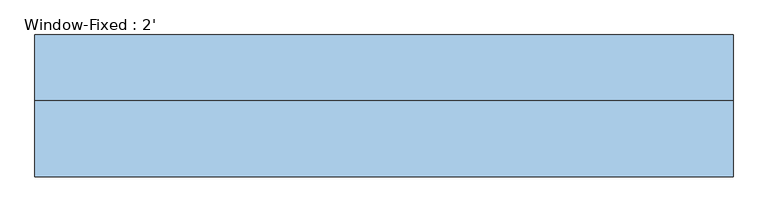
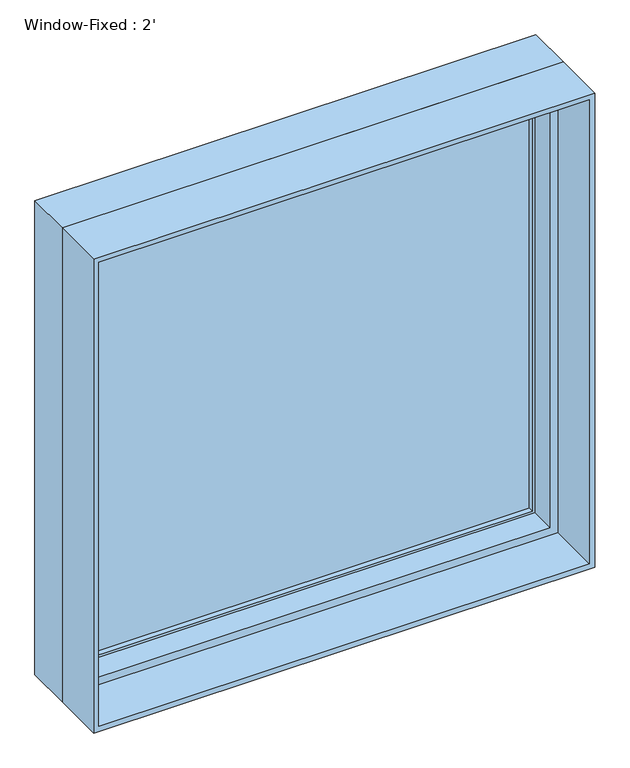
"""IFC4 building model written with IfcOpenShell, lengths in millimetres: window geometry, Window-Fixed : 2'."""

from ifc_helpers import new_model, si_unit, frame, origin, place, context, project, spatial, polyline, outline, extrude, faceted_brep, source, transform, mapped, element, save


def window_fixed_2_d4a0c5b4(model_context):
    return source(origin(), model_context, "Body", "SolidModel", [
        faceted_brep([(609.6, 19.05, 2133.6), (609.6, 133.35, 2133.6), (-609.6, 133.35, 2133.6), (-609.6, 19.05, 2133.6), (-609.6, 133.35, 914.4), (-609.6, 19.05, 914.4), (609.6, 133.35, 914.4), (609.6, 19.05, 914.4), (577.85, 19.05, 2101.85), (577.85, 19.05, 946.15), (-577.85, 19.05, 946.15), (-577.85, 19.05, 2101.85), (-596.9, 133.35, 2120.9), (-596.9, 133.35, 927.1), (596.9, 133.35, 927.1), (596.9, 133.35, 2120.9), (577.85, 82.55, 2101.85), (-577.85, 82.55, 2101.85), (596.9, 82.55, 2120.9), (-596.9, 82.55, 2120.9), (-577.85, 82.55, 946.15), (-596.9, 82.55, 927.1), (577.85, 82.55, 946.15), (596.9, 82.55, 927.1)], [[[0, 1, 2, 3]], [[3, 2, 4, 5]], [[5, 4, 6, 7]], [[3, 5, 7, 0], [8, 9, 10, 11]], [[7, 6, 1, 0]], [[1, 6, 4, 2], [12, 13, 14, 15]], [[16, 8, 11, 17]], [[15, 18, 19, 12]], [[17, 11, 10, 20]], [[12, 19, 21, 13]], [[20, 10, 9, 22]], [[13, 21, 23, 14]], [[22, 9, 8, 16]], [[18, 23, 21, 19], [17, 20, 22, 16]], [[14, 23, 18, 15]]]),
        extrude(outline(polyline([(2133.6, -609.6), (914.4, -609.6), (914.4, 609.6), (2133.6, 609.6), (2133.6, -609.6)]), holes=[polyline([(2120.9, 596.9), (927.1, 596.9), (927.1, -596.9), (2120.9, -596.9), (2120.9, 596.9)])]), frame((0.0, -114.3, 0.0), z_axis=(0.0, 1.0, 0.0), x_axis=(0.0, 0.0, 1.0)), (0.0, 0.0, 1.0), 133.35),
        extrude(outline(polyline([(927.1, 596.9), (2120.9, 596.9), (2120.9, -596.9), (927.1, -596.9), (927.1, 596.9)]), holes=[polyline([(952.5, -571.5), (2095.5, -571.5), (2095.5, 571.5), (952.5, 571.5), (952.5, -571.5)])]), frame((0.0, 82.55, 0.0), z_axis=(0.0, 1.0, 0.0), x_axis=(0.0, 0.0, 1.0)), (0.0, 0.0, 1.0), 44.45),
        extrude(outline(polyline([(571.5, 114.3), (571.5, 107.95), (-571.5, 107.95), (-571.5, 114.3), (571.5, 114.3)])), frame((0.0, 0.0, 952.5), z_axis=(0.0, 0.0, 1.0), x_axis=(1.0, 0.0, 0.0)), (0.0, 0.0, 1.0), 1143.0),
        extrude(outline(polyline([(-571.5, 95.25), (-571.5, 101.6), (571.5, 101.6), (571.5, 95.25), (-571.5, 95.25)])), frame((0.0, 0.0, 952.5), z_axis=(0.0, 0.0, 1.0), x_axis=(1.0, 0.0, 0.0)), (0.0, 0.0, 1.0), 1143.0),
    ])


if __name__ == "__main__":
    model = new_model("IFC4")
    model_context = context("Model", 3, world=origin())
    ifc_project = project(units=[si_unit("LENGTHUNIT", "METRE", prefix="MILLI")], contexts=[model_context])
    site = spatial("IfcSite", under=ifc_project)
    building = spatial("IfcBuilding", under=site)
    placement = place(None, origin())
    window_fixed_2_shape = window_fixed_2_d4a0c5b4(model_context)
    element("IfcWindow", 1, ObjectType="Window-Fixed : 2'", at=placement, inside=building, context=model_context, shape_type="MappedRepresentation", body=[
        mapped(window_fixed_2_shape, transform((0.0, 0.0, 0.0), x_axis=(1.0, 0.0, 0.0), y_axis=(0.0, 1.0, 0.0), z_axis=(0.0, 0.0, 1.0))),
    ])
    save(model, "model.ifc")

# Revit data of these elements
# Type "Window-Fixed : 2'"
#   Type Mark = "28"
#   Fire Rating = "0.5h"
#   Assembly Code = "B2020100"
#   Analytic Construction = "Double glazing - domestic"
#   Window Inset [instance default] = 0' - 0"
#   Wall Thickness [instance default] = 0' - 6"
#   Visual Light Transmittance = 0.81
#   Thermal Resistance (R) = 1.8146 (h·ft²·°F)/BTU
#   Solar Heat Gain Coefficient = 0.76
#   Rough Width = 4' - 0 1/2"
#   Rough Height = 4' - 0 1/2"
#   Interior Wall Closure [instance default] = 0' - 2 1/4"
#   Height = 4' - 0"
#   Heat Transfer Coefficient (U) = 0.5511 BTU/(h·ft²·°F)
#   Frame Extension [instance default] = 0' - 0 1/4"
#   Exterior Wall Closure [instance default] = 0' - 1 1/4"
#   Extension Jamb [instance default] = 0' - 2 1/4"
#   Default Sill Height = 3' - 0"
#   Width = 4' - 0"
#   Muntin Visibility = yes
#   Interior Trim Visibility [instance default] = yes
#   Exterior Trim Visibility [instance default] = yes
#   Extension Jamb Visibility [instance default] = yes
#   Muntin Pattern = Muntin Pattern_2x2 : Muntin Pattern_2x2
#   Interior Trim Material = Wood - Stained
#   Interior Trim = Trim-Window-Interior-Flat : Picture Frame
#   Interior Frame Material = Wood - Stained
#   Glass Panel Material = Glass
#   Exterior Trim Material = Clad - White
#   Exterior Trim = Trim-Window-Exterior-Flat : with Sill
#   Exterior Frame Material = Clad - White
#   Wall Closure = (empty or 0)
# Element 1 (IfcWindow, "Window-Fixed : 2'")
#   Wall Thickness = 0' - 9"
#   Extension Jamb = 0' - 5 1/4"
#   Materials on its faces: "Wood - Stained", "Glass", "Clad - White"
# Materials
#   "Wood - Stained": class "Wood", colour RGB 224 178 126, transparency 0, Cost = 0
#   "Glass": class "Glass", colour RGB 0 128 192, transparency 0.75, Description = "Soda Lime Glass", Cost = 0
#   "Clad - White": class "Wood", colour RGB 242 242 238, transparency 0, Cost = 0
